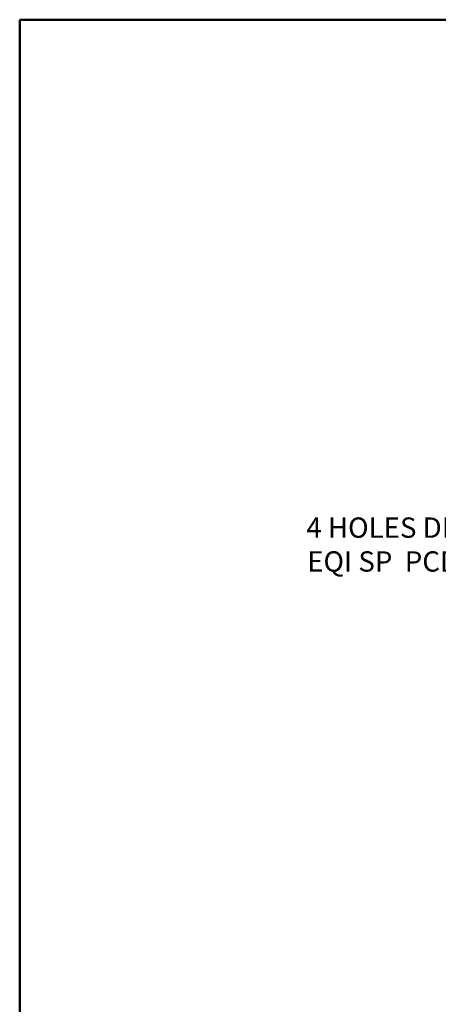
# Model space of a CAD drawing. Units: millimetres. Extents: x -166 to 681, y -4360 to 126.
# Tile 2 of 7: x -166 to -22, y -213 to 126. Entities that reach past the tile are written whole.
import ezdxf
from ezdxf import colors
from ezdxf.entities.mleader import LeaderData, LeaderLine
from ezdxf.math import Vec2, Vec3

# ---------------------------------------------------------------- set-up
doc = ezdxf.new("R2010")
doc.units = ezdxf.units.MM
doc.header["$LTSCALE"] = 0.5
doc.layers.add('M-TEXT', color=7, linetype='Continuous', lineweight=25)
doc.layers.add('M-TTLB', color=7, linetype='Continuous', lineweight=50)
doc.styles.get("Standard").update_dxf_attribs({"font": 'arial.ttf'})

msp = doc.modelspace()

# ---------------------------------------------------------------- linework, layer by layer
at = {"layer": 'M-TTLB', "ltscale": 0.5}
msp.add_lwpolyline([(-165.9437, 126.0872), (680.7907, 126.0872), (680.7907, -430.0081), (-165.9437, -430.0081)], close=True, dxfattribs=at)

# ---------------------------------------------------------------- leaders
at = {"layer": 'M-TEXT', "ltscale": 0.5}
ml = msp.add_multileader_mtext('Standard', dxfattribs=at)
ml.set_content('4 HOLES DIA 8,\\P EQI SP  PCD 56', color=256)
ml.set_leader_properties()
ml.build(insert=Vec2(0, 0))
ctx = ml.context
ctx.base_point, ctx.char_height, ctx.plane_origin = Vec3(-78.2306, -49.2827), 7, Vec3(28.8008, -13.8088)
ctx.text_align_type = 2
notes = []
notes.append((ctx, [(0, (1, 1, 0), (8.3199, -49.2827), (-1, 0), 8, [(0, [(28.8008, -13.8088)], 0, [])])]))
ctx.mtext.insert, ctx.mtext.alignment, ctx.mtext.flow_direction = Vec3(-1.6801, -45.5106), 3, 5
for ctx, leaders in notes:
    for number, flags, end, landing, length, lines in leaders:
        leader = LeaderData()
        leader.index, (leader.has_last_leader_line, leader.has_dogleg_vector, leader.attachment_direction) = number, flags
        leader.last_leader_point, leader.dogleg_vector, leader.dogleg_length = Vec3(end), Vec3(landing), length
        for number, points, colour, breaks in lines:
            line = LeaderLine()
            line.index, line.vertices, line.color, line.breaks = number, Vec3.list(points), colors.encode_raw_color(colour), breaks
            leader.lines.append(line)
        ctx.leaders.append(leader)

doc.saveas('drawing.dxf')
